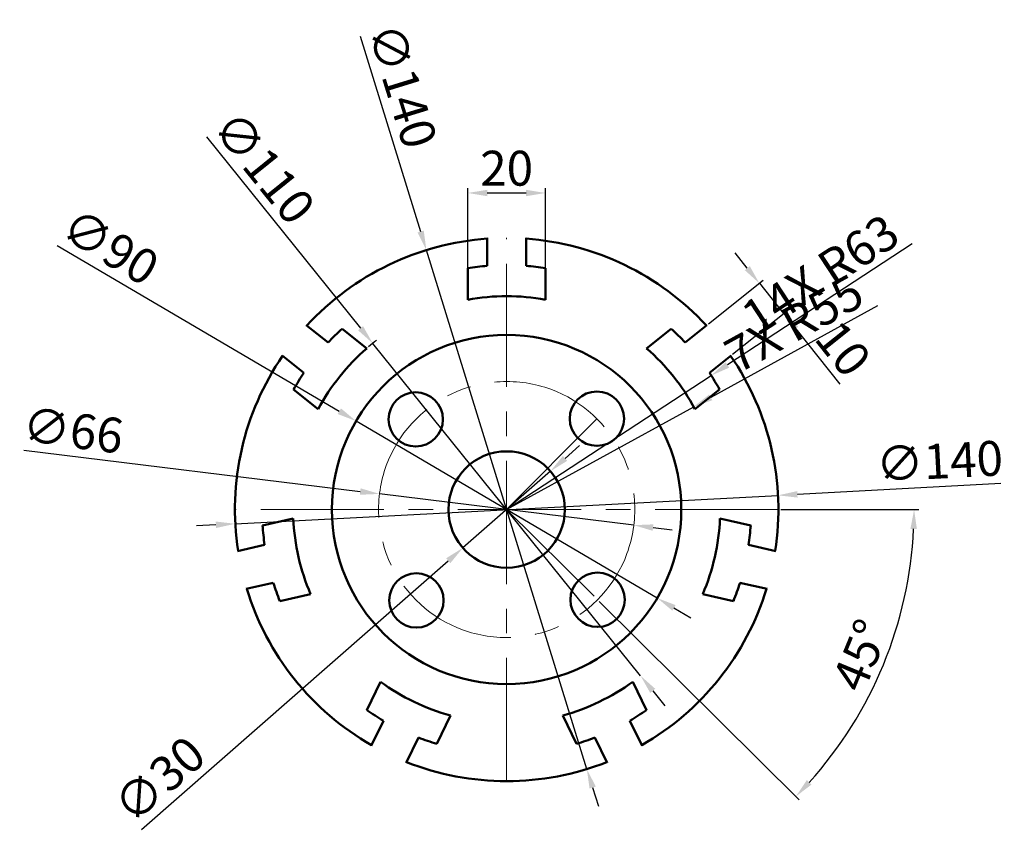
# Model space of a CAD drawing. Units: millimetres. Extents: x 2617 to 2870, y 1424 to 1633.
import ezdxf

# ---------------------------------------------------------------- set-up
doc = ezdxf.new("R2010")
doc.units = ezdxf.units.MM
doc.linetypes.add('CENTER', pattern=[50.8, 31.75, -6.35, 6.35, -6.35])
for name, color, linetype, lineweight in [('M-CNTR', 4, 'CENTER', 18), ('M-CONS', 8, 'Continuous', 13), ('M-DIMS', 2, 'Continuous', 25), ('M-OUTL', 7, 'Continuous', 50)]:
    doc.layers.add(name, color=color, linetype=linetype, lineweight=lineweight)
doc.styles.get("Standard").update_dxf_attribs({"font": 'arial.ttf'})
doc.dimstyles.new('ISO-25', dxfattribs={"dimtxt": 9, "dimasz": 5, "dimexe": 1.25, "dimexo": 0.625, "dimtad": 1, "dimtxsty": 'Standard', "dimcen": 2.5, "dimadec": 0, "dimazin": 0, "dimtfac": 1, "dimtmove": 0, "dimatfit": 3, "dimfxl": 1, "dimarcsym": 0})

# ---------------------------------------------------------------- blocks, each defined once
blk = doc.blocks.new('*D1')
at = {"layer": 'Defpoints', "color": 0, "transparency": 16777216}
for p in [(2752.24, 1588.62), (2732.24, 1561.11), (2752.24, 1561.11)]:
    blk.add_point(p, dxfattribs=at)
at = {"layer": 'M-DIMS', "color": 0, "lineweight": -2, "transparency": 16777216}
for p, q in [((2732.24, 1561.74), (2732.24, 1589.87)), ((2737.24, 1588.62), (2747.24, 1588.62)), ((2752.24, 1561.74), (2752.24, 1589.87))]:
    blk.add_line(p, q, dxfattribs=at)
at = {"layer": 'M-DIMS', "color": 0, "transparency": 16777216}
for points in [[(2737.24, 1589.45), (2737.24, 1587.79), (2732.24, 1588.62)], [(2747.24, 1589.45), (2747.24, 1587.79), (2752.24, 1588.62)]]:
    blk.add_solid(points, dxfattribs=at)
at = {"layer": 'M-DIMS', "color": 0, "transparency": 16777216, "insert": (2742.24, 1593.84), "char_height": 9, "attachment_point": 5}
blk.add_mtext('20', dxfattribs=at)
blk = doc.blocks.new('*D2')
at = {"layer": 'Defpoints', "color": 0, "transparency": 16777216}
for p in [(2813.58, 1557.53), (2793.71, 1554.47), (2799.94, 1546.65)]:
    blk.add_point(p, dxfattribs=at)
at = {"layer": 'M-DIMS', "color": 0, "lineweight": -2, "transparency": 16777216}
for p, q in [((2804.23, 1569.25), (2801.11, 1573.16)), ((2794.2, 1554.86), (2808.32, 1566.12)), ((2807.34, 1565.34), (2813.58, 1557.53)), ((2800.43, 1547.04), (2814.56, 1558.31)), ((2816.7, 1553.62), (2828.08, 1539.34))]:
    blk.add_line(p, q, dxfattribs=at)
at = {"layer": 'M-DIMS', "color": 0, "transparency": 16777216}
for points in [[(2804.88, 1569.77), (2803.58, 1568.73), (2807.34, 1565.34)], [(2817.35, 1554.14), (2816.05, 1553.1), (2813.58, 1557.53)]]:
    blk.add_solid(points, dxfattribs=at)
at = {"layer": 'M-DIMS', "color": 0, "transparency": 16777216, "insert": (2828.03, 1547.78), "char_height": 9, "attachment_point": 5, "rotation": 308.5714}
blk.add_mtext('10', dxfattribs=at)
blk = doc.blocks.new('*D3')
at = {"layer": 'Defpoints', "color": 0, "transparency": 16777216}
for p in [(2753.52, 1516.91), (2730.95, 1497.14)]:
    blk.add_point(p, dxfattribs=at)
at = {"layer": 'M-DIMS', "color": 0, "lineweight": -2, "transparency": 16777216}
for p, q in [((2757.28, 1520.21), (2761.04, 1523.5)), ((2753.52, 1516.91), (2730.95, 1497.14)), ((2648.14, 1424.57), (2727.19, 1493.85))]:
    blk.add_line(p, q, dxfattribs=at)
at = {"layer": 'M-DIMS', "color": 0, "transparency": 16777216}
for points in [[(2756.73, 1520.84), (2757.83, 1519.58), (2753.52, 1516.91)], [(2726.65, 1494.47), (2727.74, 1493.22), (2730.95, 1497.14)]]:
    blk.add_solid(points, dxfattribs=at)
at = {"layer": 'M-DIMS', "color": 0, "transparency": 16777216, "insert": (2653.52, 1436.56), "char_height": 9, "attachment_point": 5, "rotation": 41.2291}
blk.add_mtext('∅30', dxfattribs=at)
blk = doc.blocks.new('*D4')
at = {"layer": 'Defpoints', "color": 0, "transparency": 16777216}
for p in [(2709.48, 1511.06), (2774.99, 1503)]:
    blk.add_point(p, dxfattribs=at)
at = {"layer": 'M-DIMS', "color": 0, "lineweight": -2, "transparency": 16777216}
for p, q in [((2617.82, 1522.34), (2704.52, 1511.67)), ((2774.99, 1503), (2709.48, 1511.06)), ((2779.95, 1502.39), (2784.91, 1501.77))]:
    blk.add_line(p, q, dxfattribs=at)
at = {"layer": 'M-DIMS', "color": 0, "transparency": 16777216}
for points in [[(2704.62, 1512.5), (2704.42, 1510.84), (2709.48, 1511.06)], [(2780.05, 1503.21), (2779.85, 1501.56), (2774.99, 1503)]]:
    blk.add_solid(points, dxfattribs=at)
at = {"layer": 'M-DIMS', "color": 0, "transparency": 16777216, "insert": (2630.37, 1526.31), "char_height": 9, "attachment_point": 5, "rotation": 352.9829}
blk.add_mtext('∅66', dxfattribs=at)
blk = doc.blocks.new('*D5')
at = {"layer": 'Defpoints', "color": 0, "transparency": 16777216}
for p in [(2703.44, 1529.84), (2781.03, 1484.22)]:
    blk.add_point(p, dxfattribs=at)
at = {"layer": 'M-DIMS', "color": 0, "lineweight": -2, "transparency": 16777216}
for p, q in [((2626.46, 1575.1), (2699.13, 1532.37)), ((2781.03, 1484.22), (2703.44, 1529.84)), ((2785.34, 1481.68), (2789.65, 1479.15))]:
    blk.add_line(p, q, dxfattribs=at)
at = {"layer": 'M-DIMS', "color": 0, "transparency": 16777216}
for points in [[(2699.56, 1533.09), (2698.71, 1531.65), (2703.44, 1529.84)], [(2785.76, 1482.4), (2784.92, 1480.97), (2781.03, 1484.22)]]:
    blk.add_solid(points, dxfattribs=at)
at = {"layer": 'M-DIMS', "color": 0, "transparency": 16777216, "insert": (2639.54, 1573.76), "char_height": 9, "attachment_point": 5, "rotation": 329.5458}
blk.add_mtext('∅90', dxfattribs=at)
blk = doc.blocks.new('*D6')
at = {"layer": 'Defpoints', "color": 0, "transparency": 16777216}
for p in [(2707.74, 1549.87), (2776.73, 1464.19)]:
    blk.add_point(p, dxfattribs=at)
at = {"layer": 'M-DIMS', "color": 0, "lineweight": -2, "transparency": 16777216}
for p, q in [((2664.89, 1603.08), (2704.6, 1553.76)), ((2776.73, 1464.19), (2707.74, 1549.87)), ((2779.87, 1460.3), (2783, 1456.4))]:
    blk.add_line(p, q, dxfattribs=at)
blk.add_arc((2742.24, 1507.03), 55, 127.5406, 130.3018, dxfattribs=at)
at = {"layer": 'M-DIMS', "color": 0, "transparency": 16777216}
for points in [[(2705.25, 1554.28), (2703.96, 1553.24), (2707.74, 1549.87)], [(2780.52, 1460.82), (2779.22, 1459.77), (2776.73, 1464.19)]]:
    blk.add_solid(points, dxfattribs=at)
at = {"layer": 'M-DIMS', "color": 0, "transparency": 16777216, "insert": (2678.84, 1594.48), "char_height": 9, "attachment_point": 5, "rotation": 308.8427}
blk.add_mtext('∅110', dxfattribs=at)
blk = doc.blocks.new('*D7')
at = {"layer": 'Defpoints', "color": 0, "transparency": 16777216}
for p in [(2721.56, 1573.9), (2762.91, 1440.15)]:
    blk.add_point(p, dxfattribs=at)
at = {"layer": 'M-DIMS', "color": 0, "lineweight": -2, "transparency": 16777216}
for p, q in [((2704.51, 1629.06), (2720.08, 1578.68)), ((2762.91, 1440.15), (2721.56, 1573.9)), ((2764.39, 1435.37), (2765.87, 1430.6))]:
    blk.add_line(p, q, dxfattribs=at)
at = {"layer": 'M-DIMS', "color": 0, "transparency": 16777216}
for points in [[(2720.88, 1578.93), (2719.29, 1578.43), (2721.56, 1573.9)], [(2765.19, 1435.62), (2763.59, 1435.13), (2762.91, 1440.15)]]:
    blk.add_solid(points, dxfattribs=at)
at = {"layer": 'M-DIMS', "color": 0, "transparency": 16777216, "insert": (2714.3, 1615.91), "char_height": 9, "attachment_point": 5, "rotation": 287.1806}
blk.add_mtext('∅140', dxfattribs=at)
blk = doc.blocks.new('*D8')
at = {"layer": 'Defpoints', "color": 0, "transparency": 16777216}
for p in [(2672.24, 1507.03), (2742.24, 1507.03), (2812.24, 1507.03), (2765.66, 1483.78), (2833.28, 1454.77)]:
    blk.add_point(p, dxfattribs=at)
at = {"layer": 'M-DIMS', "color": 0, "lineweight": -2, "transparency": 16777216}
for p, q in [((2812.86, 1507.03), (2848.46, 1507.03)), ((2766.1, 1483.34), (2817.63, 1432.2))]:
    blk.add_line(p, q, dxfattribs=at)
blk.add_arc((2742.24, 1507.03), 104.97, 317.9455, 357.2706, dxfattribs=at)
at = {"layer": 'M-DIMS', "color": 0, "transparency": 16777216}
for points in [[(2846.26, 1502.05), (2847.92, 1502.01), (2847.21, 1507.03)], [(2820.78, 1436.14), (2819.57, 1437.29), (2816.74, 1433.08)]]:
    blk.add_solid(points, dxfattribs=at)
at = {"layer": 'M-DIMS', "color": 0, "transparency": 16777216, "insert": (2834.48, 1469.02), "char_height": 9, "attachment_point": 5, "rotation": 67.6081}
blk.add_mtext('45°', dxfattribs=at)
blk = doc.blocks.new('FLANGE-RADIAL-T-SLOT')
for p, q in [((5, 8.72), (5, 15.92)), ((15, 8.72), (15, 15.92)), ((0, 0), (0, 8.12)), ((20, 0), (20, 8.12))]:
    blk.add_line(p, q)
for radius, start, end in [(63, 94.5521, 99.1332), (63, 80.8668, 85.4479), (55, 79.5243, 100.4757)]:
    blk.add_arc((10, -54.08), radius, start, end)
blk = doc.blocks.new('MOUNTING-HOLE-D14')
blk.add_circle((7, 7), 7)
blk = doc.blocks.new('*D11')
at = {"layer": 'Defpoints', "color": 0, "transparency": 16777216}
for p in [(2812.14, 1510.69), (2672.33, 1503.36)]:
    blk.add_point(p, dxfattribs=at)
at = {"layer": 'M-DIMS', "color": 0, "lineweight": -2, "transparency": 16777216}
for p, q in [((2869.51, 1513.7), (2817.13, 1510.95)), ((2672.33, 1503.36), (2812.14, 1510.69)), ((2667.34, 1503.1), (2662.35, 1502.84))]:
    blk.add_line(p, q, dxfattribs=at)
at = {"layer": 'M-DIMS', "color": 0, "transparency": 16777216}
for points in [[(2817.09, 1511.78), (2817.18, 1510.12), (2812.14, 1510.69)], [(2667.3, 1503.94), (2667.38, 1502.27), (2672.33, 1503.36)]]:
    blk.add_solid(points, dxfattribs=at)
at = {"layer": 'M-DIMS', "color": 0, "transparency": 16777216, "insert": (2853.8, 1518.35), "char_height": 9, "attachment_point": 5, "rotation": 2.9993}
blk.add_mtext('∅140', dxfattribs=at)
blk = doc.blocks.new('*D12')
at = {"layer": 'Defpoints', "color": 0, "transparency": 16777216}
for p in [(2794.93, 1541.56), (2742.24, 1507.03)]:
    blk.add_point(p, dxfattribs=at)
at = {"layer": 'M-DIMS', "color": 0, "lineweight": -2, "transparency": 16777216}
for p, q in [((2846.72, 1575.5), (2799.11, 1544.3)), ((2742.24, 1507.03), (2794.93, 1541.56))]:
    blk.add_line(p, q, dxfattribs=at)
at = {"layer": 'M-DIMS', "color": 0, "transparency": 16777216}
blk.add_solid([(2798.65, 1545), (2799.57, 1543.6), (2794.93, 1541.56)], dxfattribs=at)
at = {"layer": 'M-DIMS', "color": 0, "transparency": 16777216, "insert": (2823.68, 1566.65), "char_height": 9, "attachment_point": 5, "rotation": 33.2386}
blk.add_mtext('14X R63', dxfattribs=at)
blk = doc.blocks.new('*D13')
at = {"layer": 'Defpoints', "color": 0, "transparency": 16777216}
for p in [(2790.43, 1533.53), (2742.24, 1507.03)]:
    blk.add_point(p, dxfattribs=at)
at = {"layer": 'M-DIMS', "color": 0, "lineweight": -2, "transparency": 16777216}
for p, q in [((2837.79, 1559.57), (2794.81, 1535.94)), ((2742.24, 1507.03), (2790.43, 1533.53))]:
    blk.add_line(p, q, dxfattribs=at)
at = {"layer": 'M-DIMS', "color": 0, "transparency": 16777216}
blk.add_solid([(2794.41, 1536.67), (2795.21, 1535.21), (2790.43, 1533.53)], dxfattribs=at)
at = {"layer": 'M-DIMS', "color": 0, "transparency": 16777216, "insert": (2816.84, 1553.99), "char_height": 9, "attachment_point": 5, "rotation": 28.8071}
blk.add_mtext('7X R55', dxfattribs=at)

msp = doc.modelspace()

# ---------------------------------------------------------------- linework, layer by layer
at = {"layer": 'M-CNTR'}
for p, q in [((2742.236, 1437.027), (2742.236, 1577.027)), ((2812.236, 1507.027), (2672.236, 1507.027)), ((2742.236, 1507.027), (2765.658, 1483.781))]:
    msp.add_line(p, q, dxfattribs=at)
msp.add_circle((2742.236, 1507.027), 33, dxfattribs=at)
at = {"layer": 'M-CONS'}
msp.add_line((2742.236, 1507.027), (2765.482, 1530.45), dxfattribs=at)
at = {"layer": 'M-OUTL'}
for radius in [45, 15]:
    msp.add_circle((2742.236, 1507.027), radius, dxfattribs=at)
for start, end in [(94.09604, 137.33253), (42.66747, 85.90396), (145.52462, 188.7611), (351.2389, 34.47538), (196.95319, 240.18967), (299.81033, 343.04681), (248.38176, 291.61824)]:
    msp.add_arc((2742.236, 1507.027), 70, start, end, dxfattribs=at)

# ---------------------------------------------------------------- block references
for name, p in [('FLANGE-RADIAL-T-SLOT', (2732.236, 1561.111)), ('MOUNTING-HOLE-D14', (2711.813, 1523.274)), ('MOUNTING-HOLE-D14', (2758.482, 1523.45)), ('MOUNTING-HOLE-D14', (2711.989, 1476.605)), ('MOUNTING-HOLE-D14', (2758.658, 1476.781))]:
    msp.add_blockref(name, p, dxfattribs=at)
for p, rotation in [((2693.717, 1532.93), 51.42857142857113), ((2778.285, 1548.566), 308.5714285714282), ((2691.733, 1485.243), 102.8571428571432), ((2797.189, 1504.742), 257.1428571428575), ((2727.78, 1453.961), 154.2857142857148), ((2774.712, 1462.638), 205.7142857142852)]:
    msp.add_blockref('FLANGE-RADIAL-T-SLOT', p, dxfattribs=dict(at, rotation=rotation))

# ---------------------------------------------------------------- dimensions: what is measured, and where the dimension line sits
at = {"layer": 'M-DIMS'}
for p1, p2, override, picture, middle in [((2762.913, 1440.151), (2721.559, 1573.904), {"dimclrd": 0, "dimclre": 0, "dimclrt": 0}, '*D7', (2709.07, 1614.299)), ((2776.731, 1464.189), (2707.741, 1549.865), {"dimclrd": 0, "dimclre": 0, "dimclrt": 0}, '*D6', (2674.579, 1591.048)), ((2781.028, 1484.219), (2703.444, 1529.836), {"dimclrd": 0, "dimclre": 0, "dimclrt": 0}, '*D5', (2636.763, 1569.042)), ((2774.989, 1502.996), (2709.483, 1511.059), {"dimclrd": 0, "dimclre": 0, "dimclrt": 0}, '*D4', (2629.699, 1520.879)), ((2672.332, 1503.365), (2812.14, 1510.69), {"dimdec": 0, "dimlfac": 1, "dimrnd": 0, "dimzin": 0, "dimdsep": 46, "dimlunit": 2}, '*D11', (2854.083, 1512.888)), ((2753.517, 1516.913), (2730.955, 1497.141), {"dimclrd": 0, "dimclre": 0, "dimclrt": 0}, '*D3', (2657.125, 1432.442))]:
    dim = msp.add_diameter_dim_2p(p1=p1, p2=p2, dimstyle='ISO-25', override=override, dxfattribs=at)
    dim.commit()
    dim.dimension.update_dxf_attribs({"geometry": picture, "text_midpoint": middle, "dimtype": 163})
dim = msp.add_linear_dim(base=(2752.236, 1588.618), p1=(2732.236, 1561.111), p2=(2752.236, 1561.111), dimstyle='ISO-25', override={"dimclrd": 0, "dimclre": 0, "dimclrt": 0}, dxfattribs=at)
dim.commit()
dim.dimension.update_dxf_attribs({"geometry": '*D1', "text_midpoint": (2742.236, 1593.839)})
for mpoint, text, picture, middle in [((2794.929, 1541.559), '14X <>', '*D12', (2826.545, 1562.278)), ((2790.43, 1533.53), '7X <>', '*D13', (2819.346, 1549.431))]:
    dim = msp.add_radius_dim(center=(2742.236, 1507.027), mpoint=mpoint, text=text, dimstyle='ISO-25', override={"dimdec": 0, "dimlfac": 1, "dimrnd": 0, "dimzin": 0, "dimdsep": 46, "dimlunit": 2}, dxfattribs=at)
    dim.commit()
    dim.dimension.update_dxf_attribs({"geometry": picture, "text_midpoint": middle, "dimtype": 164})
dim = msp.add_aligned_dim(p1=(2793.707, 1554.469), p2=(2799.942, 1546.651), distance=17.443, dimstyle='ISO-25', override={"dimclrd": 0, "dimclre": 0, "dimclrt": 0}, dxfattribs=at)
dim.commit()
dim.dimension.update_dxf_attribs({"geometry": '*D2', "text_midpoint": (2828.031, 1547.778)})
dim = msp.add_angular_dim_2l(base=(2833.276, 1454.77), line1=((2812.236, 1507.027), (2672.236, 1507.027)), line2=((2742.236, 1507.027), (2765.658, 1483.781)), dimstyle='ISO-25', override={"dimclrd": 0, "dimclre": 0, "dimclrt": 0}, dxfattribs=at)
dim.commit()
dim.dimension.update_dxf_attribs({"geometry": '*D8', "text_midpoint": (2834.484, 1469.021)})

doc.saveas('drawing.dxf')
